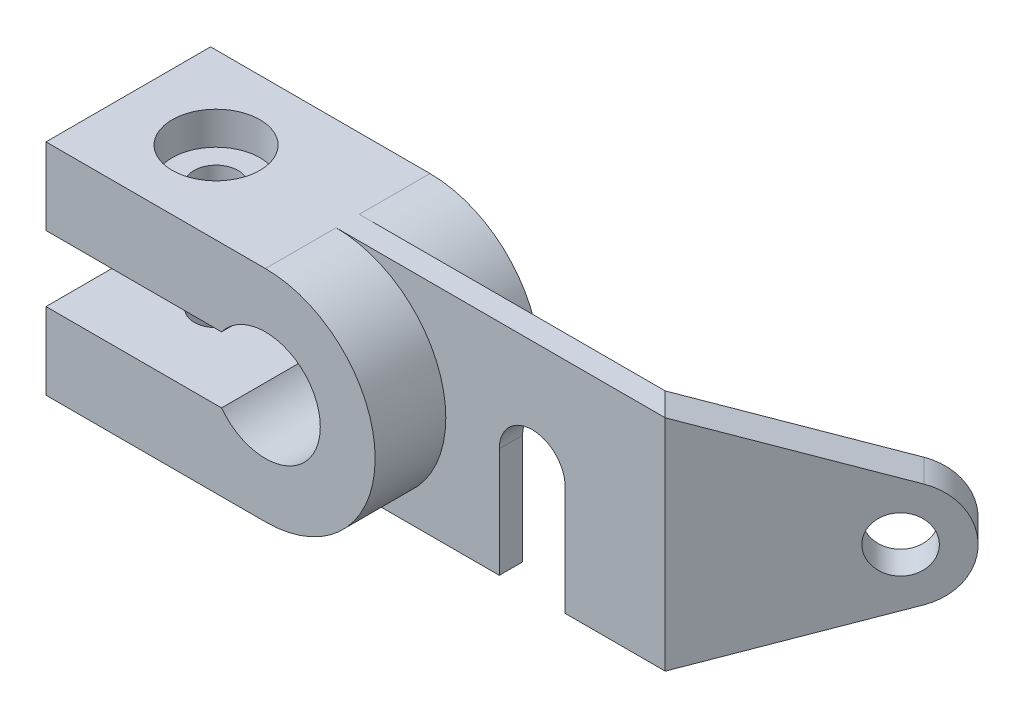
ISO-10303-21;
HEADER;
FILE_DESCRIPTION(('STEP AP214'),'2;1');
FILE_NAME('part.step','',(''),(''),'','','');
FILE_SCHEMA(('AUTOMOTIVE_DESIGN { 1 0 10303 214 1 1 1 1 }'));
ENDSEC;
DATA;
#1=APPLICATION_CONTEXT('core data for automotive mechanical design processes');
#2=APPLICATION_PROTOCOL_DEFINITION('international standard','automotive_design',2000,#1);
#3=PRODUCT_CONTEXT('',#1,'mechanical');
#4=PRODUCT('Part','Part','',(#3));
#5=PRODUCT_RELATED_PRODUCT_CATEGORY('part','',(#4));
#6=PRODUCT_DEFINITION_FORMATION('','',#4);
#7=PRODUCT_DEFINITION_CONTEXT('part definition',#1,'design');
#8=PRODUCT_DEFINITION('design','',#6,#7);
#9=PRODUCT_DEFINITION_SHAPE('','',#8);
#10=(LENGTH_UNIT() NAMED_UNIT(*) SI_UNIT(.MILLI.,.METRE.));
#11=(NAMED_UNIT(*) PLANE_ANGLE_UNIT() SI_UNIT($,.RADIAN.));
#12=(NAMED_UNIT(*) SI_UNIT($,.STERADIAN.) SOLID_ANGLE_UNIT());
#13=UNCERTAINTY_MEASURE_WITH_UNIT(LENGTH_MEASURE(1.E-05),#10,'distance_accuracy_value','');
#14=(GEOMETRIC_REPRESENTATION_CONTEXT(3) GLOBAL_UNCERTAINTY_ASSIGNED_CONTEXT((#13)) GLOBAL_UNIT_ASSIGNED_CONTEXT((#10,
#11,#12)) REPRESENTATION_CONTEXT('',''));
#15=CARTESIAN_POINT('',(0.,0.,0.));
#16=DIRECTION('',(0.,0.,1.));
#17=DIRECTION('',(1.,0.,0.));
#18=AXIS2_PLACEMENT_3D('',#15,#16,#17);
#19=CARTESIAN_POINT('',(6.36396103067889,60.,6.36396103067896));
#20=DIRECTION('',(-0.707106781186544,0.,-0.707106781186551));
#21=DIRECTION('',(-0.707106781186551,0.,0.707106781186544));
#22=AXIS2_PLACEMENT_3D('',#19,#20,#21);
#23=PLANE('',#22);
#24=CARTESIAN_POINT('',(38.537319574667,30.,-25.8093975133088));
#25=DIRECTION('',(-0.707106781186544,0.,-0.707106781186551));
#26=DIRECTION('',(-0.707106781186551,0.,0.707106781186544));
#27=AXIS2_PLACEMENT_3D('',#24,#25,#26);
#28=CIRCLE('',#27,7.49999999999999);
#29=CARTESIAN_POINT('',(33.2340187157678,30.,-20.5060966544097));
#30=VERTEX_POINT('',#29);
#31=EDGE_CURVE('E382',#30,#30,#28,.T.);
#32=ORIENTED_EDGE('',*,*,#31,.T.);
#33=EDGE_LOOP('',(#32));
#34=FACE_BOUND('',#33,.T.);
#35=DIRECTION('',(0.674665588129943,0.299420587780075,-0.674665588129936));
#36=VECTOR('',#35,1.);
#37=CARTESIAN_POINT('',(18.4844870478504,5.37916130319396,-5.75656498649238));
#38=LINE('',#37,#36);
#39=CARTESIAN_POINT('',(6.36396103067889,0.,6.36396103067896));
#40=VERTEX_POINT('',#39);
#41=CARTESIAN_POINT('',(41.7131544953593,15.6881816280033,-28.985232434001));
#42=VERTEX_POINT('',#41);
#43=EDGE_CURVE('E195',#40,#42,#38,.T.);
#44=ORIENTED_EDGE('',*,*,#43,.T.);
#45=CARTESIAN_POINT('',(38.537319574667,30.,-25.8093975133088));
#46=DIRECTION('',(-0.707106781186544,0.,-0.707106781186551));
#47=DIRECTION('',(-0.707106781186551,0.,0.707106781186544));
#48=AXIS2_PLACEMENT_3D('',#45,#46,#47);
#49=CIRCLE('',#48,15.);
#50=CARTESIAN_POINT('',(41.7131544953593,44.3118183719967,-28.985232434001));
#51=VERTEX_POINT('',#50);
#52=EDGE_CURVE('E364',#51,#42,#49,.T.);
#53=ORIENTED_EDGE('',*,*,#52,.F.);
#54=DIRECTION('',(-0.674665588129943,0.299420587780075,0.674665588129936));
#55=VECTOR('',#54,1.);
#56=CARTESIAN_POINT('',(6.36396103067889,60.,6.36396103067896));
#57=LINE('',#56,#55);
#58=CARTESIAN_POINT('',(6.36396103067892,60.,6.36396103067897));
#59=VERTEX_POINT('',#58);
#60=EDGE_CURVE('E361',#51,#59,#57,.T.);
#61=ORIENTED_EDGE('',*,*,#60,.T.);
#62=DIRECTION('',(0.,-1.,0.));
#63=VECTOR('',#62,1.);
#64=CARTESIAN_POINT('',(6.36396103067889,60.,6.36396103067896));
#65=LINE('',#64,#63);
#66=EDGE_CURVE('E225',#59,#40,#65,.T.);
#67=ORIENTED_EDGE('',*,*,#66,.T.);
#68=EDGE_LOOP('',(#44,#53,#61,#67));
#69=FACE_BOUND('',#68,.T.);
#70=ADVANCED_FACE('F64',(#34,#69),#23,.F.);
#71=CARTESIAN_POINT('',(0.,60.,0.));
#72=DIRECTION('',(0.707106781186544,0.,0.707106781186551));
#73=DIRECTION('',(0.707106781186551,0.,-0.707106781186544));
#74=AXIS2_PLACEMENT_3D('',#71,#72,#73);
#75=PLANE('',#74);
#76=CARTESIAN_POINT('',(32.1733585439881,30.,-32.1733585439877));
#77=DIRECTION('',(-0.707106781186544,0.,-0.707106781186551));
#78=DIRECTION('',(-0.707106781186551,0.,0.707106781186544));
#79=AXIS2_PLACEMENT_3D('',#76,#77,#78);
#80=CIRCLE('',#79,7.49999999999999);
#81=CARTESIAN_POINT('',(26.8700576850889,30.,-26.8700576850887));
#82=VERTEX_POINT('',#81);
#83=EDGE_CURVE('E381',#82,#82,#80,.T.);
#84=ORIENTED_EDGE('',*,*,#83,.F.);
#85=EDGE_LOOP('',(#84));
#86=FACE_BOUND('',#85,.T.);
#87=CARTESIAN_POINT('',(32.1733585439881,30.,-32.1733585439877));
#88=DIRECTION('',(-0.707106781186544,0.,-0.707106781186551));
#89=DIRECTION('',(-0.707106781186551,0.,0.707106781186544));
#90=AXIS2_PLACEMENT_3D('',#87,#88,#89);
#91=CIRCLE('',#90,15.);
#92=CARTESIAN_POINT('',(35.3491934646804,44.3118183719967,-35.34919346468));
#93=VERTEX_POINT('',#92);
#94=CARTESIAN_POINT('',(35.3491934646804,15.6881816280033,-35.34919346468));
#95=VERTEX_POINT('',#94);
#96=EDGE_CURVE('E208',#93,#95,#91,.T.);
#97=ORIENTED_EDGE('',*,*,#96,.T.);
#98=DIRECTION('',(0.674665588129943,0.299420587780076,-0.674665588129936));
#99=VECTOR('',#98,1.);
#100=CARTESIAN_POINT('',(0.,0.,0.));
#101=LINE('',#100,#99);
#102=CARTESIAN_POINT('',(0.,0.,0.));
#103=VERTEX_POINT('',#102);
#104=EDGE_CURVE('E194',#103,#95,#101,.T.);
#105=ORIENTED_EDGE('',*,*,#104,.F.);
#106=DIRECTION('',(0.,-1.,0.));
#107=VECTOR('',#106,1.);
#108=CARTESIAN_POINT('',(0.,60.,0.));
#109=LINE('',#108,#107);
#110=CARTESIAN_POINT('',(0.,60.,0.));
#111=VERTEX_POINT('',#110);
#112=EDGE_CURVE('E210',#111,#103,#109,.T.);
#113=ORIENTED_EDGE('',*,*,#112,.F.);
#114=DIRECTION('',(-0.674665588129943,0.299420587780075,0.674665588129936));
#115=VECTOR('',#114,1.);
#116=CARTESIAN_POINT('',(12.1205260171715,54.6208386968061,-12.1205260171713));
#117=LINE('',#116,#115);
#118=EDGE_CURVE('E391',#93,#111,#117,.T.);
#119=ORIENTED_EDGE('',*,*,#118,.F.);
#120=EDGE_LOOP('',(#97,#105,#113,#119));
#121=FACE_BOUND('',#120,.T.);
#122=ADVANCED_FACE('F203',(#86,#121),#75,.F.);
#123=CARTESIAN_POINT('',(0.,0.,0.));
#124=DIRECTION('',(0.,-1.,0.));
#125=DIRECTION('',(0.,0.,-1.));
#126=AXIS2_PLACEMENT_3D('',#123,#124,#125);
#127=PLANE('',#126);
#128=DIRECTION('',(-0.707106781186544,0.,-0.707106781186551));
#129=VECTOR('',#128,1.);
#130=CARTESIAN_POINT('',(86.9741340859449,0.,86.9741340859458));
#131=LINE('',#130,#129);
#132=EDGE_CURVE('E186',#40,#103,#131,.T.);
#133=ORIENTED_EDGE('',*,*,#132,.F.);
#134=DIRECTION('',(1.,0.,0.));
#135=VECTOR('',#134,1.);
#136=CARTESIAN_POINT('',(6.36396103067889,0.,6.36396103067896));
#137=LINE('',#136,#135);
#138=CARTESIAN_POINT('',(-21.,0.,6.36396103067896));
#139=VERTEX_POINT('',#138);
#140=EDGE_CURVE('E217',#139,#40,#137,.T.);
#141=ORIENTED_EDGE('',*,*,#140,.F.);
#142=DIRECTION('',(0.,0.,-1.));
#143=VECTOR('',#142,1.);
#144=CARTESIAN_POINT('',(-21.,0.,0.));
#145=LINE('',#144,#143);
#146=CARTESIAN_POINT('',(-21.,0.,0.));
#147=VERTEX_POINT('',#146);
#148=EDGE_CURVE('E216',#139,#147,#145,.T.);
#149=ORIENTED_EDGE('',*,*,#148,.T.);
#150=DIRECTION('',(-1.,0.,0.));
#151=VECTOR('',#150,1.);
#152=CARTESIAN_POINT('',(-48.3863389600815,0.,0.));
#153=LINE('',#152,#151);
#154=EDGE_CURVE('E213',#103,#147,#153,.T.);
#155=ORIENTED_EDGE('',*,*,#154,.F.);
#156=EDGE_LOOP('',(#133,#141,#149,#155));
#157=FACE_BOUND('',#156,.T.);
#158=ADVANCED_FACE('F215',(#157),#127,.T.);
#159=CARTESIAN_POINT('',(-119.636038969321,-42.,3.18198051533949));
#160=DIRECTION('',(0.,1.,0.));
#161=DIRECTION('',(0.,0.,1.));
#162=AXIS2_PLACEMENT_3D('',#159,#160,#161);
#163=CYLINDRICAL_SURFACE('',#162,6.);
#164=CARTESIAN_POINT('',(-119.636038969321,21.,3.18198051533949));
#165=DIRECTION('',(0.,-1.,0.));
#166=DIRECTION('',(0.,0.,-1.));
#167=AXIS2_PLACEMENT_3D('',#164,#165,#166);
#168=CIRCLE('',#167,6.);
#169=CARTESIAN_POINT('',(-119.636038969321,21.,-2.81801948466051));
#170=VERTEX_POINT('',#169);
#171=EDGE_CURVE('E242',#170,#170,#168,.F.);
#172=ORIENTED_EDGE('',*,*,#171,.T.);
#173=EDGE_LOOP('',(#172));
#174=FACE_BOUND('',#173,.T.);
#175=CARTESIAN_POINT('',(-119.636038969321,9.,3.18198051533949));
#176=DIRECTION('',(0.,-1.,0.));
#177=DIRECTION('',(0.,0.,-1.));
#178=AXIS2_PLACEMENT_3D('',#175,#176,#177);
#179=CIRCLE('',#178,6.);
#180=CARTESIAN_POINT('',(-119.636038969321,9.,-2.81801948466051));
#181=VERTEX_POINT('',#180);
#182=EDGE_CURVE('E253',#181,#181,#179,.T.);
#183=ORIENTED_EDGE('',*,*,#182,.T.);
#184=EDGE_LOOP('',(#183));
#185=FACE_BOUND('',#184,.T.);
#186=ADVANCED_FACE('F450',(#174,#185),#163,.F.);
#187=CARTESIAN_POINT('',(-119.636038969321,30.,3.18198051533949));
#188=DIRECTION('',(0.,1.,0.));
#189=DIRECTION('',(0.,0.,1.));
#190=AXIS2_PLACEMENT_3D('',#187,#188,#189);
#191=CYLINDRICAL_SURFACE('',#190,6.);
#192=CARTESIAN_POINT('',(-119.636038969321,39.,3.18198051533949));
#193=DIRECTION('',(0.,1.,0.));
#194=DIRECTION('',(0.,0.,1.));
#195=AXIS2_PLACEMENT_3D('',#192,#193,#194);
#196=CIRCLE('',#195,6.);
#197=CARTESIAN_POINT('',(-119.636038969321,39.,9.18198051533949));
#198=VERTEX_POINT('',#197);
#199=EDGE_CURVE('E247',#198,#198,#196,.F.);
#200=ORIENTED_EDGE('',*,*,#199,.T.);
#201=EDGE_LOOP('',(#200));
#202=FACE_BOUND('',#201,.T.);
#203=CARTESIAN_POINT('',(-119.636038969321,51.,3.18198051533949));
#204=DIRECTION('',(0.,1.,0.));
#205=DIRECTION('',(0.,0.,1.));
#206=AXIS2_PLACEMENT_3D('',#203,#204,#205);
#207=CIRCLE('',#206,6.);
#208=CARTESIAN_POINT('',(-119.636038969321,51.,9.18198051533949));
#209=VERTEX_POINT('',#208);
#210=EDGE_CURVE('E252',#209,#209,#207,.T.);
#211=ORIENTED_EDGE('',*,*,#210,.T.);
#212=EDGE_LOOP('',(#211));
#213=FACE_BOUND('',#212,.T.);
#214=ADVANCED_FACE('F451',(#202,#213),#191,.F.);
#215=CARTESIAN_POINT('',(-143.636038969321,0.,-19.3180194846605));
#216=DIRECTION('',(-1.,0.,0.));
#217=DIRECTION('',(0.,0.,1.));
#218=AXIS2_PLACEMENT_3D('',#215,#216,#217);
#219=PLANE('',#218);
#220=DIRECTION('',(0.,0.,1.));
#221=VECTOR('',#220,1.);
#222=CARTESIAN_POINT('',(-143.636038969321,21.,-61.3180194846605));
#223=LINE('',#222,#221);
#224=CARTESIAN_POINT('',(-143.636038969321,21.,-19.3180194846605));
#225=VERTEX_POINT('',#224);
#226=CARTESIAN_POINT('',(-143.636038969321,21.,25.6819805153395));
#227=VERTEX_POINT('',#226);
#228=EDGE_CURVE('E303',#225,#227,#223,.T.);
#229=ORIENTED_EDGE('',*,*,#228,.F.);
#230=DIRECTION('',(0.,1.,0.));
#231=VECTOR('',#230,1.);
#232=CARTESIAN_POINT('',(-143.636038969321,0.,-19.3180194846605));
#233=LINE('',#232,#231);
#234=CARTESIAN_POINT('',(-143.636038969321,0.,-19.3180194846605));
#235=VERTEX_POINT('',#234);
#236=EDGE_CURVE('E344',#235,#225,#233,.T.);
#237=ORIENTED_EDGE('',*,*,#236,.F.);
#238=DIRECTION('',(0.,0.,1.));
#239=VECTOR('',#238,1.);
#240=CARTESIAN_POINT('',(-143.636038969321,0.,-19.3180194846605));
#241=LINE('',#240,#239);
#242=CARTESIAN_POINT('',(-143.636038969321,0.,25.6819805153395));
#243=VERTEX_POINT('',#242);
#244=EDGE_CURVE('E321',#235,#243,#241,.T.);
#245=ORIENTED_EDGE('',*,*,#244,.T.);
#246=DIRECTION('',(0.,1.,0.));
#247=VECTOR('',#246,1.);
#248=CARTESIAN_POINT('',(-143.636038969321,0.,25.6819805153395));
#249=LINE('',#248,#247);
#250=EDGE_CURVE('E336',#243,#227,#249,.T.);
#251=ORIENTED_EDGE('',*,*,#250,.T.);
#252=EDGE_LOOP('',(#229,#237,#245,#251));
#253=FACE_BOUND('',#252,.T.);
#254=ADVANCED_FACE('F432',(#253),#219,.T.);
#255=CARTESIAN_POINT('',(-83.6360389693211,30.,-19.3180194846605));
#256=DIRECTION('',(0.,0.,1.));
#257=DIRECTION('',(1.,0.,0.));
#258=AXIS2_PLACEMENT_3D('',#255,#256,#257);
#259=CYLINDRICAL_SURFACE('',#258,30.);
#260=DIRECTION('',(0.,0.,-1.));
#261=VECTOR('',#260,1.);
#262=CARTESIAN_POINT('',(-83.6360389693211,0.,-19.3180194846605));
#263=LINE('',#262,#261);
#264=CARTESIAN_POINT('',(-83.6360389693211,0.,0.));
#265=VERTEX_POINT('',#264);
#266=CARTESIAN_POINT('',(-83.6360389693211,0.,-19.3180194846605));
#267=VERTEX_POINT('',#266);
#268=EDGE_CURVE('E319',#265,#267,#263,.T.);
#269=ORIENTED_EDGE('',*,*,#268,.T.);
#270=CARTESIAN_POINT('',(-83.6360389693211,30.,-19.3180194846605));
#271=DIRECTION('',(0.,0.,-1.));
#272=DIRECTION('',(-1.,0.,0.));
#273=AXIS2_PLACEMENT_3D('',#270,#271,#272);
#274=CIRCLE('',#273,30.);
#275=CARTESIAN_POINT('',(-83.6360389693211,60.,-19.3180194846605));
#276=VERTEX_POINT('',#275);
#277=EDGE_CURVE('E347',#276,#267,#274,.T.);
#278=ORIENTED_EDGE('',*,*,#277,.F.);
#279=DIRECTION('',(0.,0.,-1.));
#280=VECTOR('',#279,1.);
#281=CARTESIAN_POINT('',(-83.6360389693211,60.,-19.3180194846605));
#282=LINE('',#281,#280);
#283=CARTESIAN_POINT('',(-83.6360389693211,60.,0.));
#284=VERTEX_POINT('',#283);
#285=EDGE_CURVE('E313',#284,#276,#282,.T.);
#286=ORIENTED_EDGE('',*,*,#285,.F.);
#287=CARTESIAN_POINT('',(-83.6360389693211,30.,0.));
#288=DIRECTION('',(0.,0.,1.));
#289=DIRECTION('',(1.,0.,0.));
#290=AXIS2_PLACEMENT_3D('',#287,#288,#289);
#291=CIRCLE('',#290,30.);
#292=EDGE_CURVE('E353',#284,#265,#291,.F.);
#293=ORIENTED_EDGE('',*,*,#292,.T.);
#294=EDGE_LOOP('',(#269,#278,#286,#293));
#295=FACE_BOUND('',#294,.T.);
#296=ADVANCED_FACE('F426',(#295),#259,.T.);
#297=CARTESIAN_POINT('',(-83.6360389693211,0.,25.6819805153395));
#298=VERTEX_POINT('',#297);
#299=CARTESIAN_POINT('',(-83.6360389693211,0.,6.36396103067896));
#300=VERTEX_POINT('',#299);
#301=EDGE_CURVE('E314',#298,#300,#263,.T.);
#302=ORIENTED_EDGE('',*,*,#301,.T.);
#303=CARTESIAN_POINT('',(-83.6360389693211,30.,6.36396103067897));
#304=DIRECTION('',(0.,0.,-1.));
#305=DIRECTION('',(-1.,0.,0.));
#306=AXIS2_PLACEMENT_3D('',#303,#304,#305);
#307=CIRCLE('',#306,30.);
#308=CARTESIAN_POINT('',(-83.6360389693211,60.,6.36396103067897));
#309=VERTEX_POINT('',#308);
#310=EDGE_CURVE('E351',#300,#309,#307,.F.);
#311=ORIENTED_EDGE('',*,*,#310,.T.);
#312=CARTESIAN_POINT('',(-83.6360389693211,60.,25.6819805153395));
#313=VERTEX_POINT('',#312);
#314=EDGE_CURVE('E327',#313,#309,#282,.T.);
#315=ORIENTED_EDGE('',*,*,#314,.F.);
#316=CARTESIAN_POINT('',(-83.6360389693211,30.,25.6819805153395));
#317=DIRECTION('',(0.,0.,-1.));
#318=DIRECTION('',(-1.,0.,0.));
#319=AXIS2_PLACEMENT_3D('',#316,#317,#318);
#320=CIRCLE('',#319,30.);
#321=EDGE_CURVE('E341',#313,#298,#320,.T.);
#322=ORIENTED_EDGE('',*,*,#321,.T.);
#323=EDGE_LOOP('',(#302,#311,#315,#322));
#324=FACE_BOUND('',#323,.T.);
#325=ADVANCED_FACE('F375',(#324),#259,.T.);
#326=CARTESIAN_POINT('',(-48.3863389600815,60.,0.));
#327=DIRECTION('',(0.,0.,1.));
#328=DIRECTION('',(1.,0.,0.));
#329=AXIS2_PLACEMENT_3D('',#326,#327,#328);
#330=PLANE('',#329);
#331=CARTESIAN_POINT('',(-30.,30.,0.));
#332=DIRECTION('',(0.,0.,1.));
#333=DIRECTION('',(1.,0.,0.));
#334=AXIS2_PLACEMENT_3D('',#331,#332,#333);
#335=CIRCLE('',#334,9.00000000000001);
#336=CARTESIAN_POINT('',(-39.,30.,0.));
#337=VERTEX_POINT('',#336);
#338=CARTESIAN_POINT('',(-21.,30.,0.));
#339=VERTEX_POINT('',#338);
#340=EDGE_CURVE('E286',#337,#339,#335,.F.);
#341=ORIENTED_EDGE('',*,*,#340,.F.);
#342=DIRECTION('',(0.,-1.,0.));
#343=VECTOR('',#342,1.);
#344=CARTESIAN_POINT('',(-39.,60.,0.));
#345=LINE('',#344,#343);
#346=CARTESIAN_POINT('',(-39.,0.,0.));
#347=VERTEX_POINT('',#346);
#348=EDGE_CURVE('E279',#337,#347,#345,.T.);
#349=ORIENTED_EDGE('',*,*,#348,.T.);
#350=EDGE_CURVE('E218',#347,#265,#153,.T.);
#351=ORIENTED_EDGE('',*,*,#350,.T.);
#352=ORIENTED_EDGE('',*,*,#292,.F.);
#353=DIRECTION('',(-1.,0.,0.));
#354=VECTOR('',#353,1.);
#355=CARTESIAN_POINT('',(0.,60.,0.));
#356=LINE('',#355,#354);
#357=EDGE_CURVE('E223',#111,#284,#356,.T.);
#358=ORIENTED_EDGE('',*,*,#357,.F.);
#359=ORIENTED_EDGE('',*,*,#112,.T.);
#360=ORIENTED_EDGE('',*,*,#154,.T.);
#361=DIRECTION('',(0.,-1.,0.));
#362=VECTOR('',#361,1.);
#363=CARTESIAN_POINT('',(-21.,60.,0.));
#364=LINE('',#363,#362);
#365=EDGE_CURVE('E76',#339,#147,#364,.T.);
#366=ORIENTED_EDGE('',*,*,#365,.F.);
#367=EDGE_LOOP('',(#341,#349,#351,#352,#358,#359,#360,#366));
#368=FACE_BOUND('',#367,.T.);
#369=ADVANCED_FACE('F65',(#368),#330,.F.);
#370=CARTESIAN_POINT('',(6.36396103067889,60.,6.36396103067896));
#371=DIRECTION('',(0.,0.,-1.));
#372=DIRECTION('',(-1.,0.,0.));
#373=AXIS2_PLACEMENT_3D('',#370,#371,#372);
#374=PLANE('',#373);
#375=CARTESIAN_POINT('',(-39.,0.,6.36396103067896));
#376=VERTEX_POINT('',#375);
#377=EDGE_CURVE('E234',#300,#376,#137,.T.);
#378=ORIENTED_EDGE('',*,*,#377,.T.);
#379=DIRECTION('',(0.,1.,0.));
#380=VECTOR('',#379,1.);
#381=CARTESIAN_POINT('',(-39.,60.,6.36396103067897));
#382=LINE('',#381,#380);
#383=CARTESIAN_POINT('',(-39.,30.,6.36396103067896));
#384=VERTEX_POINT('',#383);
#385=EDGE_CURVE('E273',#376,#384,#382,.T.);
#386=ORIENTED_EDGE('',*,*,#385,.T.);
#387=CARTESIAN_POINT('',(-30.,30.,6.36396103067896));
#388=DIRECTION('',(0.,0.,-1.));
#389=DIRECTION('',(-1.,0.,0.));
#390=AXIS2_PLACEMENT_3D('',#387,#388,#389);
#391=CIRCLE('',#390,9.00000000000001);
#392=CARTESIAN_POINT('',(-21.,30.,6.36396103067896));
#393=VERTEX_POINT('',#392);
#394=EDGE_CURVE('E71',#393,#384,#391,.F.);
#395=ORIENTED_EDGE('',*,*,#394,.F.);
#396=DIRECTION('',(0.,1.,0.));
#397=VECTOR('',#396,1.);
#398=CARTESIAN_POINT('',(-21.,60.,6.36396103067896));
#399=LINE('',#398,#397);
#400=EDGE_CURVE('E278',#139,#393,#399,.T.);
#401=ORIENTED_EDGE('',*,*,#400,.F.);
#402=ORIENTED_EDGE('',*,*,#140,.T.);
#403=ORIENTED_EDGE('',*,*,#66,.F.);
#404=DIRECTION('',(1.,0.,0.));
#405=VECTOR('',#404,1.);
#406=CARTESIAN_POINT('',(6.36396103067889,60.,6.36396103067896));
#407=LINE('',#406,#405);
#408=EDGE_CURVE('E228',#309,#59,#407,.T.);
#409=ORIENTED_EDGE('',*,*,#408,.F.);
#410=ORIENTED_EDGE('',*,*,#310,.F.);
#411=EDGE_LOOP('',(#378,#386,#395,#401,#402,#403,#409,#410));
#412=FACE_BOUND('',#411,.T.);
#413=ADVANCED_FACE('F285',(#412),#374,.F.);
#414=CARTESIAN_POINT('',(0.,60.,0.));
#415=DIRECTION('',(0.,-1.,0.));
#416=DIRECTION('',(0.,0.,-1.));
#417=AXIS2_PLACEMENT_3D('',#414,#415,#416);
#418=PLANE('',#417);
#419=CARTESIAN_POINT('',(-119.636038969321,60.,3.18198051533949));
#420=DIRECTION('',(0.,1.,0.));
#421=DIRECTION('',(0.,0.,1.));
#422=AXIS2_PLACEMENT_3D('',#419,#420,#421);
#423=CIRCLE('',#422,12.);
#424=CARTESIAN_POINT('',(-119.636038969321,60.,15.1819805153395));
#425=VERTEX_POINT('',#424);
#426=EDGE_CURVE('E259',#425,#425,#423,.T.);
#427=ORIENTED_EDGE('',*,*,#426,.F.);
#428=EDGE_LOOP('',(#427));
#429=FACE_BOUND('',#428,.T.);
#430=ORIENTED_EDGE('',*,*,#408,.T.);
#431=DIRECTION('',(-0.707106781186544,0.,-0.707106781186551));
#432=VECTOR('',#431,1.);
#433=CARTESIAN_POINT('',(0.,60.,0.));
#434=LINE('',#433,#432);
#435=EDGE_CURVE('E12',#59,#111,#434,.T.);
#436=ORIENTED_EDGE('',*,*,#435,.T.);
#437=ORIENTED_EDGE('',*,*,#357,.T.);
#438=ORIENTED_EDGE('',*,*,#285,.T.);
#439=DIRECTION('',(-1.,0.,0.));
#440=VECTOR('',#439,1.);
#441=CARTESIAN_POINT('',(-83.6360389693211,60.,-19.3180194846605));
#442=LINE('',#441,#440);
#443=CARTESIAN_POINT('',(-143.636038969321,60.,-19.3180194846605));
#444=VERTEX_POINT('',#443);
#445=EDGE_CURVE('E329',#276,#444,#442,.T.);
#446=ORIENTED_EDGE('',*,*,#445,.T.);
#447=DIRECTION('',(0.,0.,1.));
#448=VECTOR('',#447,1.);
#449=CARTESIAN_POINT('',(-143.636038969321,60.,-19.3180194846605));
#450=LINE('',#449,#448);
#451=CARTESIAN_POINT('',(-143.636038969321,60.,25.6819805153395));
#452=VERTEX_POINT('',#451);
#453=EDGE_CURVE('E334',#444,#452,#450,.T.);
#454=ORIENTED_EDGE('',*,*,#453,.T.);
#455=DIRECTION('',(1.,0.,0.));
#456=VECTOR('',#455,1.);
#457=CARTESIAN_POINT('',(-83.6360389693211,60.,25.6819805153395));
#458=LINE('',#457,#456);
#459=EDGE_CURVE('E337',#452,#313,#458,.T.);
#460=ORIENTED_EDGE('',*,*,#459,.T.);
#461=ORIENTED_EDGE('',*,*,#314,.T.);
#462=EDGE_LOOP('',(#430,#436,#437,#438,#446,#454,#460,#461));
#463=FACE_BOUND('',#462,.T.);
#464=ADVANCED_FACE('F367',(#429,#463),#418,.F.);
#465=DIRECTION('',(0.,0.,-1.));
#466=VECTOR('',#465,1.);
#467=CARTESIAN_POINT('',(-39.,0.,0.));
#468=LINE('',#467,#466);
#469=EDGE_CURVE('E261',#376,#347,#468,.T.);
#470=ORIENTED_EDGE('',*,*,#469,.F.);
#471=ORIENTED_EDGE('',*,*,#377,.F.);
#472=ORIENTED_EDGE('',*,*,#301,.F.);
#473=DIRECTION('',(1.,0.,0.));
#474=VECTOR('',#473,1.);
#475=CARTESIAN_POINT('',(-83.6360389693211,0.,25.6819805153395));
#476=LINE('',#475,#474);
#477=EDGE_CURVE('E323',#243,#298,#476,.T.);
#478=ORIENTED_EDGE('',*,*,#477,.F.);
#479=ORIENTED_EDGE('',*,*,#244,.F.);
#480=DIRECTION('',(-1.,0.,0.));
#481=VECTOR('',#480,1.);
#482=CARTESIAN_POINT('',(-83.6360389693211,0.,-19.3180194846605));
#483=LINE('',#482,#481);
#484=EDGE_CURVE('E320',#267,#235,#483,.T.);
#485=ORIENTED_EDGE('',*,*,#484,.F.);
#486=ORIENTED_EDGE('',*,*,#268,.F.);
#487=ORIENTED_EDGE('',*,*,#350,.F.);
#488=EDGE_LOOP('',(#470,#471,#472,#478,#479,#485,#486,#487));
#489=FACE_BOUND('',#488,.T.);
#490=CARTESIAN_POINT('',(-119.636038969321,0.,3.18198051533949));
#491=DIRECTION('',(0.,-1.,0.));
#492=DIRECTION('',(0.,0.,-1.));
#493=AXIS2_PLACEMENT_3D('',#490,#491,#492);
#494=CIRCLE('',#493,12.);
#495=CARTESIAN_POINT('',(-119.636038969321,0.,-8.81801948466051));
#496=VERTEX_POINT('',#495);
#497=EDGE_CURVE('E292',#496,#496,#494,.T.);
#498=ORIENTED_EDGE('',*,*,#497,.F.);
#499=EDGE_LOOP('',(#498));
#500=FACE_BOUND('',#499,.T.);
#501=ADVANCED_FACE('F376',(#489,#500),#127,.T.);
#502=CARTESIAN_POINT('',(-83.6360389693211,30.,-19.3180194846605));
#503=DIRECTION('',(0.,0.,-1.));
#504=DIRECTION('',(-1.,0.,0.));
#505=AXIS2_PLACEMENT_3D('',#502,#503,#504);
#506=PLANE('',#505);
#507=DIRECTION('',(-1.,0.,0.));
#508=VECTOR('',#507,1.);
#509=CARTESIAN_POINT('',(-83.6360389693211,21.,-19.3180194846605));
#510=LINE('',#509,#508);
#511=CARTESIAN_POINT('',(-95.6360389693211,21.,-19.3180194846605));
#512=VERTEX_POINT('',#511);
#513=EDGE_CURVE('E239',#512,#225,#510,.T.);
#514=ORIENTED_EDGE('',*,*,#513,.F.);
#515=CARTESIAN_POINT('',(-83.6360389693211,30.,-19.3180194846605));
#516=DIRECTION('',(0.,0.,-1.));
#517=DIRECTION('',(-1.,0.,0.));
#518=AXIS2_PLACEMENT_3D('',#515,#516,#517);
#519=CIRCLE('',#518,15.);
#520=CARTESIAN_POINT('',(-95.6360389693211,39.,-19.3180194846605));
#521=VERTEX_POINT('',#520);
#522=EDGE_CURVE('E237',#512,#521,#519,.F.);
#523=ORIENTED_EDGE('',*,*,#522,.T.);
#524=DIRECTION('',(1.,0.,0.));
#525=VECTOR('',#524,1.);
#526=CARTESIAN_POINT('',(-83.6360389693211,39.,-19.3180194846605));
#527=LINE('',#526,#525);
#528=CARTESIAN_POINT('',(-143.636038969321,39.,-19.3180194846605));
#529=VERTEX_POINT('',#528);
#530=EDGE_CURVE('E308',#529,#521,#527,.T.);
#531=ORIENTED_EDGE('',*,*,#530,.F.);
#532=EDGE_CURVE('E330',#529,#444,#233,.T.);
#533=ORIENTED_EDGE('',*,*,#532,.T.);
#534=ORIENTED_EDGE('',*,*,#445,.F.);
#535=ORIENTED_EDGE('',*,*,#277,.T.);
#536=ORIENTED_EDGE('',*,*,#484,.T.);
#537=ORIENTED_EDGE('',*,*,#236,.T.);
#538=EDGE_LOOP('',(#514,#523,#531,#533,#534,#535,#536,#537));
#539=FACE_BOUND('',#538,.T.);
#540=ADVANCED_FACE('F440',(#539),#506,.T.);
#541=CARTESIAN_POINT('',(-83.6360389693211,30.,25.6819805153395));
#542=DIRECTION('',(0.,0.,-1.));
#543=DIRECTION('',(-1.,0.,0.));
#544=AXIS2_PLACEMENT_3D('',#541,#542,#543);
#545=PLANE('',#544);
#546=CARTESIAN_POINT('',(-83.6360389693211,30.,25.6819805153395));
#547=DIRECTION('',(0.,0.,-1.));
#548=DIRECTION('',(-1.,0.,0.));
#549=AXIS2_PLACEMENT_3D('',#546,#547,#548);
#550=CIRCLE('',#549,15.);
#551=CARTESIAN_POINT('',(-95.6360389693211,21.,25.6819805153395));
#552=VERTEX_POINT('',#551);
#553=CARTESIAN_POINT('',(-95.6360389693211,39.,25.6819805153395));
#554=VERTEX_POINT('',#553);
#555=EDGE_CURVE('E236',#552,#554,#550,.F.);
#556=ORIENTED_EDGE('',*,*,#555,.F.);
#557=DIRECTION('',(-1.,0.,0.));
#558=VECTOR('',#557,1.);
#559=CARTESIAN_POINT('',(-83.6360389693211,21.,25.6819805153395));
#560=LINE('',#559,#558);
#561=EDGE_CURVE('E86',#552,#227,#560,.T.);
#562=ORIENTED_EDGE('',*,*,#561,.T.);
#563=ORIENTED_EDGE('',*,*,#250,.F.);
#564=ORIENTED_EDGE('',*,*,#477,.T.);
#565=ORIENTED_EDGE('',*,*,#321,.F.);
#566=ORIENTED_EDGE('',*,*,#459,.F.);
#567=CARTESIAN_POINT('',(-143.636038969321,39.,25.6819805153395));
#568=VERTEX_POINT('',#567);
#569=EDGE_CURVE('E342',#568,#452,#249,.T.);
#570=ORIENTED_EDGE('',*,*,#569,.F.);
#571=DIRECTION('',(1.,0.,0.));
#572=VECTOR('',#571,1.);
#573=CARTESIAN_POINT('',(-83.6360389693211,39.,25.6819805153395));
#574=LINE('',#573,#572);
#575=EDGE_CURVE('E304',#568,#554,#574,.T.);
#576=ORIENTED_EDGE('',*,*,#575,.T.);
#577=EDGE_LOOP('',(#556,#562,#563,#564,#565,#566,#570,#576));
#578=FACE_BOUND('',#577,.T.);
#579=ADVANCED_FACE('F444',(#578),#545,.F.);
#580=DIRECTION('',(0.,0.,1.));
#581=VECTOR('',#580,1.);
#582=CARTESIAN_POINT('',(-143.636038969321,39.,-61.3180194846605));
#583=LINE('',#582,#581);
#584=EDGE_CURVE('E250',#529,#568,#583,.T.);
#585=ORIENTED_EDGE('',*,*,#584,.T.);
#586=ORIENTED_EDGE('',*,*,#569,.T.);
#587=ORIENTED_EDGE('',*,*,#453,.F.);
#588=ORIENTED_EDGE('',*,*,#532,.F.);
#589=EDGE_LOOP('',(#585,#586,#587,#588));
#590=FACE_BOUND('',#589,.T.);
#591=ADVANCED_FACE('F476',(#590),#219,.T.);
#592=CARTESIAN_POINT('',(-83.6360389693211,30.,-64.3180194846605));
#593=DIRECTION('',(0.,0.,1.));
#594=DIRECTION('',(1.,0.,0.));
#595=AXIS2_PLACEMENT_3D('',#592,#593,#594);
#596=CYLINDRICAL_SURFACE('',#595,15.);
#597=DIRECTION('',(0.,0.,1.));
#598=VECTOR('',#597,1.);
#599=CARTESIAN_POINT('',(-95.6360389693211,21.,-64.3180194846605));
#600=LINE('',#599,#598);
#601=EDGE_CURVE('E245',#552,#512,#600,.F.);
#602=ORIENTED_EDGE('',*,*,#601,.F.);
#603=ORIENTED_EDGE('',*,*,#555,.T.);
#604=DIRECTION('',(0.,0.,1.));
#605=VECTOR('',#604,1.);
#606=CARTESIAN_POINT('',(-95.6360389693211,39.,-64.3180194846605));
#607=LINE('',#606,#605);
#608=EDGE_CURVE('E230',#521,#554,#607,.T.);
#609=ORIENTED_EDGE('',*,*,#608,.F.);
#610=ORIENTED_EDGE('',*,*,#522,.F.);
#611=EDGE_LOOP('',(#602,#603,#609,#610));
#612=FACE_BOUND('',#611,.T.);
#613=ADVANCED_FACE('F466',(#612),#596,.F.);
#614=CARTESIAN_POINT('',(0.,39.,-61.3180194846605));
#615=DIRECTION('',(0.,1.,0.));
#616=DIRECTION('',(0.,0.,1.));
#617=AXIS2_PLACEMENT_3D('',#614,#615,#616);
#618=PLANE('',#617);
#619=ORIENTED_EDGE('',*,*,#199,.F.);
#620=EDGE_LOOP('',(#619));
#621=FACE_BOUND('',#620,.T.);
#622=ORIENTED_EDGE('',*,*,#530,.T.);
#623=ORIENTED_EDGE('',*,*,#608,.T.);
#624=ORIENTED_EDGE('',*,*,#575,.F.);
#625=ORIENTED_EDGE('',*,*,#584,.F.);
#626=EDGE_LOOP('',(#622,#623,#624,#625));
#627=FACE_BOUND('',#626,.T.);
#628=ADVANCED_FACE('F463',(#621,#627),#618,.F.);
#629=CARTESIAN_POINT('',(0.,21.,-61.3180194846605));
#630=DIRECTION('',(0.,-1.,0.));
#631=DIRECTION('',(0.,0.,-1.));
#632=AXIS2_PLACEMENT_3D('',#629,#630,#631);
#633=PLANE('',#632);
#634=ORIENTED_EDGE('',*,*,#171,.F.);
#635=EDGE_LOOP('',(#634));
#636=FACE_BOUND('',#635,.T.);
#637=ORIENTED_EDGE('',*,*,#513,.T.);
#638=ORIENTED_EDGE('',*,*,#228,.T.);
#639=ORIENTED_EDGE('',*,*,#561,.F.);
#640=ORIENTED_EDGE('',*,*,#601,.T.);
#641=EDGE_LOOP('',(#637,#638,#639,#640));
#642=FACE_BOUND('',#641,.T.);
#643=ADVANCED_FACE('F470',(#636,#642),#633,.F.);
#644=CARTESIAN_POINT('',(-119.636038969321,51.,3.18198051533949));
#645=DIRECTION('',(0.,1.,0.));
#646=DIRECTION('',(0.,0.,1.));
#647=AXIS2_PLACEMENT_3D('',#644,#645,#646);
#648=CYLINDRICAL_SURFACE('',#647,12.);
#649=CARTESIAN_POINT('',(-119.636038969321,51.,3.18198051533949));
#650=DIRECTION('',(0.,1.,0.));
#651=DIRECTION('',(0.,0.,1.));
#652=AXIS2_PLACEMENT_3D('',#649,#650,#651);
#653=CIRCLE('',#652,12.);
#654=CARTESIAN_POINT('',(-119.636038969321,51.,15.1819805153395));
#655=VERTEX_POINT('',#654);
#656=EDGE_CURVE('E251',#655,#655,#653,.T.);
#657=ORIENTED_EDGE('',*,*,#656,.F.);
#658=EDGE_LOOP('',(#657));
#659=FACE_BOUND('',#658,.T.);
#660=ORIENTED_EDGE('',*,*,#426,.T.);
#661=EDGE_LOOP('',(#660));
#662=FACE_BOUND('',#661,.T.);
#663=ADVANCED_FACE('F472',(#659,#662),#648,.F.);
#664=CARTESIAN_POINT('',(-119.636038969321,51.,3.18198051533949));
#665=DIRECTION('',(0.,1.,0.));
#666=DIRECTION('',(0.,0.,1.));
#667=AXIS2_PLACEMENT_3D('',#664,#665,#666);
#668=PLANE('',#667);
#669=ORIENTED_EDGE('',*,*,#210,.F.);
#670=EDGE_LOOP('',(#669));
#671=FACE_BOUND('',#670,.T.);
#672=ORIENTED_EDGE('',*,*,#656,.T.);
#673=EDGE_LOOP('',(#672));
#674=FACE_BOUND('',#673,.T.);
#675=ADVANCED_FACE('F570',(#671,#674),#668,.T.);
#676=CARTESIAN_POINT('',(-119.636038969321,9.,3.18198051533949));
#677=DIRECTION('',(0.,-1.,0.));
#678=DIRECTION('',(0.,0.,-1.));
#679=AXIS2_PLACEMENT_3D('',#676,#677,#678);
#680=CYLINDRICAL_SURFACE('',#679,12.);
#681=CARTESIAN_POINT('',(-119.636038969321,9.,3.18198051533949));
#682=DIRECTION('',(0.,-1.,0.));
#683=DIRECTION('',(0.,0.,-1.));
#684=AXIS2_PLACEMENT_3D('',#681,#682,#683);
#685=CIRCLE('',#684,12.);
#686=CARTESIAN_POINT('',(-119.636038969321,9.,-8.81801948466051));
#687=VERTEX_POINT('',#686);
#688=EDGE_CURVE('E258',#687,#687,#685,.T.);
#689=ORIENTED_EDGE('',*,*,#688,.F.);
#690=EDGE_LOOP('',(#689));
#691=FACE_BOUND('',#690,.T.);
#692=ORIENTED_EDGE('',*,*,#497,.T.);
#693=EDGE_LOOP('',(#692));
#694=FACE_BOUND('',#693,.T.);
#695=ADVANCED_FACE('F574',(#691,#694),#680,.F.);
#696=CARTESIAN_POINT('',(-119.636038969321,9.,3.18198051533949));
#697=DIRECTION('',(0.,-1.,0.));
#698=DIRECTION('',(0.,0.,-1.));
#699=AXIS2_PLACEMENT_3D('',#696,#697,#698);
#700=PLANE('',#699);
#701=ORIENTED_EDGE('',*,*,#182,.F.);
#702=EDGE_LOOP('',(#701));
#703=FACE_BOUND('',#702,.T.);
#704=ORIENTED_EDGE('',*,*,#688,.T.);
#705=EDGE_LOOP('',(#704));
#706=FACE_BOUND('',#705,.T.);
#707=ADVANCED_FACE('F587',(#703,#706),#700,.T.);
#708=CARTESIAN_POINT('',(-30.,30.,-72.));
#709=DIRECTION('',(0.,0.,1.));
#710=DIRECTION('',(1.,0.,0.));
#711=AXIS2_PLACEMENT_3D('',#708,#709,#710);
#712=CYLINDRICAL_SURFACE('',#711,9.00000000000001);
#713=ORIENTED_EDGE('',*,*,#340,.T.);
#714=DIRECTION('',(0.,0.,1.));
#715=VECTOR('',#714,1.);
#716=CARTESIAN_POINT('',(-21.,30.,-72.));
#717=LINE('',#716,#715);
#718=EDGE_CURVE('E268',#339,#393,#717,.T.);
#719=ORIENTED_EDGE('',*,*,#718,.T.);
#720=ORIENTED_EDGE('',*,*,#394,.T.);
#721=DIRECTION('',(0.,0.,1.));
#722=VECTOR('',#721,1.);
#723=CARTESIAN_POINT('',(-39.,30.,-72.));
#724=LINE('',#723,#722);
#725=EDGE_CURVE('E269',#337,#384,#724,.T.);
#726=ORIENTED_EDGE('',*,*,#725,.F.);
#727=EDGE_LOOP('',(#713,#719,#720,#726));
#728=FACE_BOUND('',#727,.T.);
#729=ADVANCED_FACE('F267',(#728),#712,.F.);
#730=CARTESIAN_POINT('',(-39.,0.,-72.));
#731=DIRECTION('',(-1.,0.,0.));
#732=DIRECTION('',(0.,0.,1.));
#733=AXIS2_PLACEMENT_3D('',#730,#731,#732);
#734=PLANE('',#733);
#735=ORIENTED_EDGE('',*,*,#725,.T.);
#736=ORIENTED_EDGE('',*,*,#385,.F.);
#737=ORIENTED_EDGE('',*,*,#469,.T.);
#738=ORIENTED_EDGE('',*,*,#348,.F.);
#739=EDGE_LOOP('',(#735,#736,#737,#738));
#740=FACE_BOUND('',#739,.T.);
#741=ADVANCED_FACE('F274',(#740),#734,.F.);
#742=CARTESIAN_POINT('',(-21.,0.,-72.));
#743=DIRECTION('',(-1.,0.,0.));
#744=DIRECTION('',(0.,-1.,0.));
#745=AXIS2_PLACEMENT_3D('',#742,#743,#744);
#746=PLANE('',#745);
#747=ORIENTED_EDGE('',*,*,#365,.T.);
#748=ORIENTED_EDGE('',*,*,#148,.F.);
#749=ORIENTED_EDGE('',*,*,#400,.T.);
#750=ORIENTED_EDGE('',*,*,#718,.F.);
#751=EDGE_LOOP('',(#747,#748,#749,#750));
#752=FACE_BOUND('',#751,.T.);
#753=ADVANCED_FACE('F379',(#752),#746,.T.);
#754=CARTESIAN_POINT('',(119.147492629933,30.,54.8007755419581));
#755=DIRECTION('',(-0.707106781186544,0.,-0.707106781186551));
#756=DIRECTION('',(-0.707106781186551,0.,0.707106781186544));
#757=AXIS2_PLACEMENT_3D('',#754,#755,#756);
#758=CYLINDRICAL_SURFACE('',#757,7.49999999999999);
#759=ORIENTED_EDGE('',*,*,#83,.T.);
#760=EDGE_LOOP('',(#759));
#761=FACE_BOUND('',#760,.T.);
#762=ORIENTED_EDGE('',*,*,#31,.F.);
#763=EDGE_LOOP('',(#762));
#764=FACE_BOUND('',#763,.T.);
#765=ADVANCED_FACE('F403',(#761,#764),#758,.F.);
#766=CARTESIAN_POINT('',(119.147492629933,30.,54.8007755419581));
#767=DIRECTION('',(-0.707106781186544,0.,-0.707106781186551));
#768=DIRECTION('',(-0.707106781186551,0.,0.707106781186544));
#769=AXIS2_PLACEMENT_3D('',#766,#767,#768);
#770=CYLINDRICAL_SURFACE('',#769,15.);
#771=ORIENTED_EDGE('',*,*,#52,.T.);
#772=DIRECTION('',(-0.707106781186544,0.,-0.707106781186551));
#773=VECTOR('',#772,1.);
#774=CARTESIAN_POINT('',(122.323327550625,15.6881816280033,51.6249406212658));
#775=LINE('',#774,#773);
#776=EDGE_CURVE('E199',#42,#95,#775,.T.);
#777=ORIENTED_EDGE('',*,*,#776,.T.);
#778=ORIENTED_EDGE('',*,*,#96,.F.);
#779=DIRECTION('',(-0.707106781186544,0.,-0.707106781186551));
#780=VECTOR('',#779,1.);
#781=CARTESIAN_POINT('',(122.323327550625,44.3118183719967,51.6249406212658));
#782=LINE('',#781,#780);
#783=EDGE_CURVE('E370',#51,#93,#782,.T.);
#784=ORIENTED_EDGE('',*,*,#783,.F.);
#785=EDGE_LOOP('',(#771,#777,#778,#784));
#786=FACE_BOUND('',#785,.T.);
#787=ADVANCED_FACE('F396',(#786),#770,.T.);
#788=CARTESIAN_POINT('',(99.0946601031163,54.6208386968061,74.8536080687745));
#789=DIRECTION('',(-0.211722328046154,-0.954121224799781,0.211722328046152));
#790=DIRECTION('',(0.976253017093471,-0.216633438360504,0.));
#791=AXIS2_PLACEMENT_3D('',#788,#789,#790);
#792=PLANE('',#791);
#793=ORIENTED_EDGE('',*,*,#783,.T.);
#794=ORIENTED_EDGE('',*,*,#118,.T.);
#795=ORIENTED_EDGE('',*,*,#435,.F.);
#796=ORIENTED_EDGE('',*,*,#60,.F.);
#797=EDGE_LOOP('',(#793,#794,#795,#796));
#798=FACE_BOUND('',#797,.T.);
#799=ADVANCED_FACE('F397',(#798),#792,.F.);
#800=CARTESIAN_POINT('',(86.9741340859449,0.,86.9741340859458));
#801=DIRECTION('',(-0.211722328046154,0.954121224799781,0.211722328046152));
#802=DIRECTION('',(-0.976253017093471,-0.216633438360504,0.));
#803=AXIS2_PLACEMENT_3D('',#800,#801,#802);
#804=PLANE('',#803);
#805=ORIENTED_EDGE('',*,*,#132,.T.);
#806=ORIENTED_EDGE('',*,*,#104,.T.);
#807=ORIENTED_EDGE('',*,*,#776,.F.);
#808=ORIENTED_EDGE('',*,*,#43,.F.);
#809=EDGE_LOOP('',(#805,#806,#807,#808));
#810=FACE_BOUND('',#809,.T.);
#811=ADVANCED_FACE('F191',(#810),#804,.F.);
#812=CLOSED_SHELL('',(#70,#122,#158,#186,#214,#254,#296,#325,#369,#413,#464,#501,#540,#579,#591,
#613,#628,#643,#663,#675,#695,#707,#729,#741,#753,#765,#787,#799,#811));
#813=MANIFOLD_SOLID_BREP('B2',#812);
#814=ADVANCED_BREP_SHAPE_REPRESENTATION('',(#18,#813),#14);
#815=SHAPE_DEFINITION_REPRESENTATION(#9,#814);
ENDSEC;
END-ISO-10303-21;
